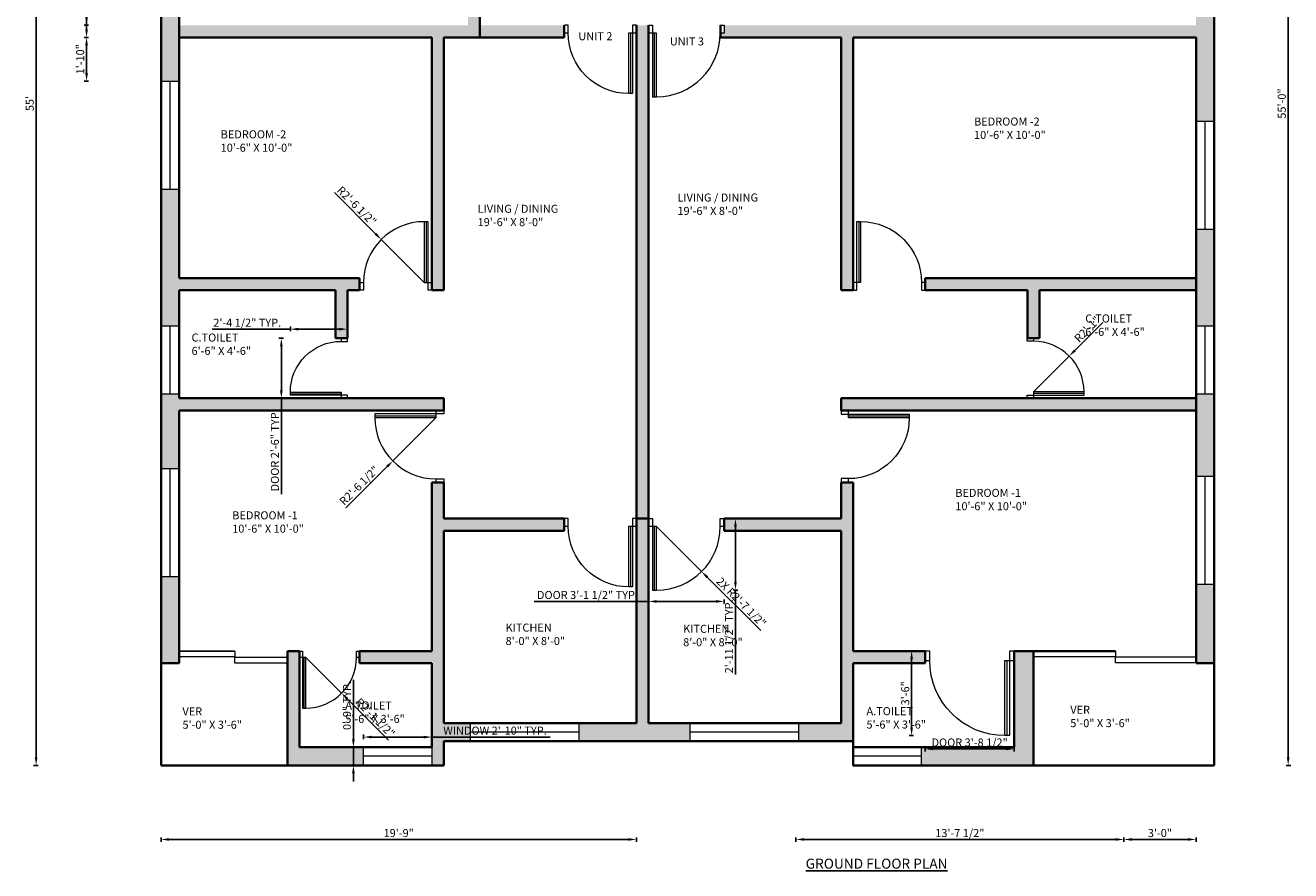
# Model space of a CAD drawing. Units: inches. Extents: x -66 to 565, y -698 to 61.
# Tile 1 of 2: x -66 to 565, y -698 to -276. Entities that reach past the tile are written whole.
import ezdxf

# ---------------------------------------------------------------- set-up
doc = ezdxf.new("R2010")
doc.units = ezdxf.units.IN
for name, color, linetype, lineweight in [('A-ANNO-DIMS', 2, 'Continuous', 18), ('A-ANNO-TEXT', 7, 'Continuous', 25), ('A-AREA-IDEN', 7, 'Continuous', 18), ('A-DOOR', 4, 'Continuous', 18), ('A-GLAZ', 111, 'Continuous', 18), ('A-WALL', 7, 'Continuous', 35), ('A-WALL-PATT', 252, 'Continuous', 13)]:
    doc.layers.add(name, color=color, linetype=linetype, lineweight=lineweight)
doc.styles.get("Standard").update_dxf_attribs({"font": 'arial.ttf'})
doc.dimstyles.new('ISO-25', dxfattribs={"dimtxt": 4, "dimasz": 4, "dimexe": 1.25, "dimexo": 0.625, "dimtad": 1, "dimlunit": 3, "dimtxsty": 'Standard', "dimcen": 2.5, "dimadec": 0, "dimazin": 0, "dimtfac": 1, "dimtmove": 0, "dimatfit": 3, "dimfxl": 1, "dimfxlon": 1, "dimarcsym": 0})

# ---------------------------------------------------------------- blocks, each defined once
blk = doc.blocks.new('A$C296830DC')
blk.add_line((829, 853), (829, 95))
for points in [[(853, 95), (853, 853), (805, 853), (805, 95)], [(47, 95), (47, 0), (0, 0), (0, 95)], [(900, 95), (900, 0), (853, 0), (853, 95)]]:
    blk.add_lwpolyline(points, close=True)
blk.add_arc((805, 95), 758, 90, 180)
blk = doc.blocks.new('*D3')
at = {"layer": 'A-ANNO-DIMS', "color": 0, "lineweight": -2, "transparency": 16777216}
for p, q in [((-59.68, 14.91), (-61.93, 14.91)), ((-60.68, 10.91), (-60.68, -641.09)), ((-59.68, -645.09), (-61.93, -645.09))]:
    blk.add_line(p, q, dxfattribs=at)
at = {"layer": 'A-ANNO-DIMS', "color": 0, "transparency": 16777216}
for points in [[(-61.35, 10.91), (-60.01, 10.91), (-60.68, 14.91)], [(-61.35, -641.09), (-60.01, -641.09), (-60.68, -645.09)]]:
    blk.add_solid(points, dxfattribs=at)
at = {"layer": 'Defpoints', "color": 0, "transparency": 16777216}
for p in [(1.61, 14.91), (-60.68, -645.09), (1.61, -645.09)]:
    blk.add_point(p, dxfattribs=at)
at = {"layer": 'A-ANNO-DIMS', "color": 0, "transparency": 16777216, "insert": (-63.34, -315.09), "char_height": 4, "attachment_point": 5, "rotation": 90}
blk.add_mtext("55'", dxfattribs=at)
blk = doc.blocks.new('WIN-54IN')
blk.add_line((4.5, 54), (4.5, 0))
blk.add_lwpolyline([(0, 54), (9, 54), (9, 0), (0, 0)], close=True)
blk = doc.blocks.new('WIN-34IN')
blk.add_line((34, 4.5), (0, 4.5))
blk.add_lwpolyline([(0, 9), (34, 9), (34, 0), (0, 0)], close=True)
blk = doc.blocks.new('*D8')
at = {"layer": 'A-ANNO-DIMS', "color": 0, "lineweight": -2, "transparency": 16777216}
for p, q in [((62.58, -432.1), (60.33, -432.1)), ((61.58, -436.1), (61.58, -458.14)), ((62.58, -462.14), (60.33, -462.14)), ((61.58, -462.14), (61.58, -509.89))]:
    blk.add_line(p, q, dxfattribs=at)
at = {"layer": 'A-ANNO-DIMS', "color": 0, "transparency": 16777216}
for points in [[(60.91, -436.1), (62.24, -436.1), (61.58, -432.1)], [(60.91, -458.14), (62.24, -458.14), (61.58, -462.14)]]:
    blk.add_solid(points, dxfattribs=at)
at = {"layer": 'Defpoints', "color": 0, "transparency": 16777216}
for p in [(66.08, -432.1), (61.58, -462.14), (66.08, -462.14)]:
    blk.add_point(p, dxfattribs=at)
at = {"layer": 'A-ANNO-DIMS', "color": 0, "transparency": 16777216, "insert": (58.88, -488.02), "char_height": 4, "attachment_point": 5, "rotation": 90}
blk.add_mtext('DOOR 2\'-6" TYP.', dxfattribs=at)
blk = doc.blocks.new('*D9')
at = {"layer": 'A-ANNO-DIMS', "color": 0, "lineweight": -2, "transparency": 16777216}
for p, q in [((66.08, -427.6), (27.06, -427.6)), ((66.08, -428.6), (66.08, -426.35)), ((90.54, -427.6), (70.08, -427.6)), ((94.54, -428.6), (94.54, -426.35))]:
    blk.add_line(p, q, dxfattribs=at)
at = {"layer": 'A-ANNO-DIMS', "color": 0, "transparency": 16777216}
for points in [[(70.08, -426.93), (70.08, -428.27), (66.08, -427.6)], [(90.54, -426.93), (90.54, -428.27), (94.54, -427.6)]]:
    blk.add_solid(points, dxfattribs=at)
at = {"layer": 'Defpoints', "color": 0, "transparency": 16777216}
for p in [(66.08, -427.6), (66.08, -432.1), (94.54, -432.1)]:
    blk.add_point(p, dxfattribs=at)
at = {"layer": 'A-ANNO-DIMS', "color": 0, "transparency": 16777216, "insert": (44.57, -424.91), "char_height": 4, "attachment_point": 5}
blk.add_mtext('2\'-4 1/2" TYP.', dxfattribs=at)
blk = doc.blocks.new('*D12')
at = {"layer": 'A-ANNO-DIMS', "color": 0, "lineweight": -2, "transparency": 16777216}
for p, q in [((244.73, -563.36), (187.66, -563.36)), ((244.73, -562.36), (244.73, -564.61)), ((278.34, -563.36), (248.73, -563.36)), ((282.34, -562.36), (282.34, -564.61))]:
    blk.add_line(p, q, dxfattribs=at)
at = {"layer": 'A-ANNO-DIMS', "color": 0, "transparency": 16777216}
for points in [[(248.73, -562.69), (248.73, -564.03), (244.73, -563.36)], [(278.34, -562.69), (278.34, -564.03), (282.34, -563.36)]]:
    blk.add_solid(points, dxfattribs=at)
at = {"layer": 'Defpoints', "color": 0, "transparency": 16777216}
for p in [(244.73, -557.72), (282.34, -557.72), (244.73, -563.36)]:
    blk.add_point(p, dxfattribs=at)
at = {"layer": 'A-ANNO-DIMS', "color": 0, "transparency": 16777216, "insert": (214.2, -560.66), "char_height": 4, "attachment_point": 5}
blk.add_mtext('DOOR 3\'-1 1/2" TYP.', dxfattribs=at)
blk = doc.blocks.new('*D13')
at = {"layer": 'A-ANNO-DIMS', "color": 0, "lineweight": -2, "transparency": 16777216}
for p, q in [((286.98, -522.09), (289.23, -522.09)), ((287.98, -526.09), (287.98, -553.72)), ((286.98, -557.72), (289.23, -557.72)), ((287.98, -557.72), (287.98, -599.85))]:
    blk.add_line(p, q, dxfattribs=at)
at = {"layer": 'A-ANNO-DIMS', "color": 0, "transparency": 16777216}
for points in [[(287.32, -526.09), (288.65, -526.09), (287.98, -522.09)], [(287.32, -553.72), (288.65, -553.72), (287.98, -557.72)]]:
    blk.add_solid(points, dxfattribs=at)
at = {"layer": 'Defpoints', "color": 0, "transparency": 16777216}
for p in [(282.34, -522.09), (282.34, -557.72), (287.98, -557.72)]:
    blk.add_point(p, dxfattribs=at)
at = {"layer": 'A-ANNO-DIMS', "color": 0, "transparency": 16777216, "insert": (285.29, -580.78), "char_height": 4, "attachment_point": 5, "rotation": 90}
blk.add_mtext('2\'-11 1/2" TYP.', dxfattribs=at)
blk = doc.blocks.new('*D14')
at = {"layer": 'A-ANNO-DIMS', "color": 0, "lineweight": -2, "transparency": 16777216}
for p, q in [((382.5, -635.91), (382.5, -638.16)), ((386.5, -636.91), (422.99, -636.91)), ((426.99, -635.91), (426.99, -638.16))]:
    blk.add_line(p, q, dxfattribs=at)
at = {"layer": 'A-ANNO-DIMS', "color": 0, "transparency": 16777216}
for points in [[(386.5, -636.24), (386.5, -637.58), (382.5, -636.91)], [(422.99, -636.24), (422.99, -637.58), (426.99, -636.91)]]:
    blk.add_solid(points, dxfattribs=at)
at = {"layer": 'Defpoints', "color": 0, "transparency": 16777216}
for p in [(382.5, -630.24), (426.99, -630.24), (426.99, -636.91)]:
    blk.add_point(p, dxfattribs=at)
at = {"layer": 'A-ANNO-DIMS', "color": 0, "transparency": 16777216, "insert": (404.74, -634.21), "char_height": 4, "attachment_point": 5}
blk.add_mtext('DOOR 3\'-8 1/2"', dxfattribs=at)
blk = doc.blocks.new('*D15')
at = {"layer": 'A-ANNO-DIMS', "color": 0, "lineweight": -2, "transparency": 16777216}
for p, q in [((376.82, -588.09), (374.57, -588.09)), ((375.82, -592.09), (375.82, -626.24)), ((376.82, -630.24), (374.57, -630.24))]:
    blk.add_line(p, q, dxfattribs=at)
at = {"layer": 'A-ANNO-DIMS', "color": 0, "transparency": 16777216}
for points in [[(375.16, -592.09), (376.49, -592.09), (375.82, -588.09)], [(375.16, -626.24), (376.49, -626.24), (375.82, -630.24)]]:
    blk.add_solid(points, dxfattribs=at)
at = {"layer": 'Defpoints', "color": 0, "transparency": 16777216}
for p in [(382.5, -588.09), (375.82, -630.24), (382.5, -630.24)]:
    blk.add_point(p, dxfattribs=at)
at = {"layer": 'A-ANNO-DIMS', "color": 0, "transparency": 16777216, "insert": (373.15, -609.16), "char_height": 4, "attachment_point": 5, "rotation": 90}
blk.add_mtext('3\'-6"', dxfattribs=at)
blk = doc.blocks.new('*D18')
at = {"layer": 'A-ANNO-DIMS', "color": 0, "lineweight": -2, "transparency": 16777216}
for p, q in [((102.6, -631.99), (102.6, -629.74)), ((136.6, -631.99), (136.6, -629.74)), ((106.6, -630.99), (132.6, -630.99)), ((136.6, -630.99), (195.57, -630.99))]:
    blk.add_line(p, q, dxfattribs=at)
at = {"layer": 'A-ANNO-DIMS', "color": 0, "transparency": 16777216}
for points in [[(106.6, -630.32), (106.6, -631.65), (102.6, -630.99)], [(132.6, -630.32), (132.6, -631.65), (136.6, -630.99)]]:
    blk.add_solid(points, dxfattribs=at)
at = {"layer": 'Defpoints', "color": 0, "transparency": 16777216}
for p in [(102.6, -636.09), (136.6, -630.99), (136.6, -636.09)]:
    blk.add_point(p, dxfattribs=at)
at = {"layer": 'A-ANNO-DIMS', "color": 0, "transparency": 16777216, "insert": (168.09, -628.29), "char_height": 4, "attachment_point": 5}
blk.add_mtext('WINDOW 2\'-10" TYP.', dxfattribs=at)
blk = doc.blocks.new('*D19')
at = {"layer": 'A-ANNO-DIMS', "color": 0, "lineweight": -2, "transparency": 16777216}
for p, q in [((97.5, -632.09), (97.5, -602.45)), ((98.5, -636.09), (96.25, -636.09)), ((97.5, -645.09), (97.5, -636.09)), ((98.5, -645.09), (96.25, -645.09)), ((97.5, -649.09), (97.5, -653.09))]:
    blk.add_line(p, q, dxfattribs=at)
at = {"layer": 'A-ANNO-DIMS', "color": 0, "transparency": 16777216}
for points in [[(96.83, -632.09), (98.17, -632.09), (97.5, -636.09)], [(96.83, -649.09), (98.17, -649.09), (97.5, -645.09)]]:
    blk.add_solid(points, dxfattribs=at)
at = {"layer": 'Defpoints', "color": 0, "transparency": 16777216}
for p in [(97.5, -636.09), (102.6, -636.09), (102.6, -645.09)]:
    blk.add_point(p, dxfattribs=at)
at = {"layer": 'A-ANNO-DIMS', "color": 0, "transparency": 16777216, "insert": (94.83, -615.27), "char_height": 4, "attachment_point": 5, "rotation": 90}
blk.add_mtext('0\'-9" TYP.', dxfattribs=at)
blk = doc.blocks.new('*D21')
at = {"layer": 'A-ANNO-DIMS', "color": 0, "lineweight": -2, "transparency": 16777216}
for p, q in [((562.56, 14.91), (564.81, 14.91)), ((563.56, 10.91), (563.56, -641.09)), ((562.56, -645.09), (564.81, -645.09))]:
    blk.add_line(p, q, dxfattribs=at)
at = {"layer": 'A-ANNO-DIMS', "color": 0, "transparency": 16777216}
for points in [[(562.89, 10.91), (564.23, 10.91), (563.56, 14.91)], [(562.89, -641.09), (564.23, -641.09), (563.56, -645.09)]]:
    blk.add_solid(points, dxfattribs=at)
at = {"layer": 'Defpoints', "color": 0, "transparency": 16777216}
for p in [(481.61, 14.91), (526.61, -645.09), (563.56, -645.09)]:
    blk.add_point(p, dxfattribs=at)
at = {"layer": 'A-ANNO-DIMS', "color": 0, "transparency": 16777216, "insert": (560.89, -315.09), "char_height": 4, "attachment_point": 5, "rotation": 90}
blk.add_mtext('55\'-0"', dxfattribs=at)
blk = doc.blocks.new('*D22')
at = {"layer": 'A-ANNO-DIMS', "color": 0, "lineweight": -2, "transparency": 16777216}
for p, q in [((-34.52, 14.91), (-36.77, 14.91)), ((-35.52, 10.91), (-35.52, -278.09)), ((-34.52, -282.09), (-36.77, -282.09))]:
    blk.add_line(p, q, dxfattribs=at)
at = {"layer": 'A-ANNO-DIMS', "color": 0, "transparency": 16777216}
for points in [[(-36.19, 10.91), (-34.86, 10.91), (-35.52, 14.91)], [(-36.19, -278.09), (-34.86, -278.09), (-35.52, -282.09)]]:
    blk.add_solid(points, dxfattribs=at)
at = {"layer": 'Defpoints', "color": 0, "transparency": 16777216}
for p in [(1.61, 14.91), (-35.52, -282.09), (10.61, -282.09)]:
    blk.add_point(p, dxfattribs=at)
at = {"layer": 'A-ANNO-DIMS', "color": 0, "transparency": 16777216, "insert": (-38.19, -133.59), "char_height": 4, "attachment_point": 5, "rotation": 90}
blk.add_mtext('24\'-9"', dxfattribs=at)
blk = doc.blocks.new('*D23')
at = {"layer": 'A-ANNO-DIMS', "color": 0, "lineweight": -2, "transparency": 16777216}
for p, q in [((1.61, -681.04), (1.61, -683.29)), ((238.61, -681.04), (238.61, -683.29)), ((5.61, -682.04), (234.61, -682.04))]:
    blk.add_line(p, q, dxfattribs=at)
at = {"layer": 'A-ANNO-DIMS', "color": 0, "transparency": 16777216}
for points in [[(5.61, -681.37), (5.61, -682.7), (1.61, -682.04)], [(234.61, -681.37), (234.61, -682.7), (238.61, -682.04)]]:
    blk.add_solid(points, dxfattribs=at)
at = {"layer": 'Defpoints', "color": 0, "transparency": 16777216}
for p in [(238.61, -624.09), (1.61, -645.09), (238.61, -682.04)]:
    blk.add_point(p, dxfattribs=at)
at = {"layer": 'A-ANNO-DIMS', "color": 0, "transparency": 16777216, "insert": (120.11, -679.37), "char_height": 4, "attachment_point": 5}
blk.add_mtext('19\'-9"', dxfattribs=at)
blk = doc.blocks.new('*D24')
at = {"layer": 'A-ANNO-DIMS', "color": 0, "lineweight": -2, "transparency": 16777216}
for p, q in [((-34.52, -186.09), (-36.77, -186.09)), ((-35.52, -190.09), (-35.52, -272.09)), ((-34.52, -276.09), (-36.77, -276.09))]:
    blk.add_line(p, q, dxfattribs=at)
at = {"layer": 'A-ANNO-DIMS', "color": 0, "transparency": 16777216}
for points in [[(-36.19, -190.09), (-34.86, -190.09), (-35.52, -186.09)], [(-36.19, -272.09), (-34.86, -272.09), (-35.52, -276.09)]]:
    blk.add_solid(points, dxfattribs=at)
at = {"layer": 'Defpoints', "color": 0, "transparency": 16777216}
for p in [(318.11, -186.09), (-35.52, -276.09), (318.11, -276.09)]:
    blk.add_point(p, dxfattribs=at)
at = {"layer": 'A-ANNO-DIMS', "color": 0, "transparency": 16777216, "insert": (-38.19, -231.09), "char_height": 4, "attachment_point": 5, "rotation": 90}
blk.add_mtext('7\'-6"', dxfattribs=at)
blk = doc.blocks.new('*D25')
at = {"layer": 'A-ANNO-DIMS', "color": 0, "lineweight": -2, "transparency": 16777216}
for p, q in [((318.11, -681.04), (318.11, -683.29)), ((481.61, -681.04), (481.61, -683.29)), ((322.11, -682.04), (477.61, -682.04))]:
    blk.add_line(p, q, dxfattribs=at)
at = {"layer": 'A-ANNO-DIMS', "color": 0, "transparency": 16777216}
for points in [[(322.11, -681.37), (322.11, -682.7), (318.11, -682.04)], [(477.61, -681.37), (477.61, -682.7), (481.61, -682.04)]]:
    blk.add_solid(points, dxfattribs=at)
at = {"layer": 'Defpoints', "color": 0, "transparency": 16777216}
for p in [(318.11, -276.09), (481.61, -276.09), (481.61, -682.04)]:
    blk.add_point(p, dxfattribs=at)
at = {"layer": 'A-ANNO-DIMS', "color": 0, "transparency": 16777216, "insert": (399.86, -679.34), "char_height": 4, "attachment_point": 5}
blk.add_mtext('13\'-7 1/2"', dxfattribs=at)
blk = doc.blocks.new('*D26')
at = {"layer": 'A-ANNO-DIMS', "color": 0, "lineweight": -2, "transparency": 16777216}
for p, q in [((481.61, -681.04), (481.61, -683.29)), ((517.61, -681.04), (517.61, -683.29)), ((513.61, -682.04), (485.61, -682.04))]:
    blk.add_line(p, q, dxfattribs=at)
at = {"layer": 'A-ANNO-DIMS', "color": 0, "transparency": 16777216}
for points in [[(485.61, -681.37), (485.61, -682.7), (481.61, -682.04)], [(513.61, -681.37), (513.61, -682.7), (517.61, -682.04)]]:
    blk.add_solid(points, dxfattribs=at)
at = {"layer": 'Defpoints', "color": 0, "transparency": 16777216}
for p in [(481.61, -276.09), (517.61, -276.09), (481.61, -682.04)]:
    blk.add_point(p, dxfattribs=at)
at = {"layer": 'A-ANNO-DIMS', "color": 0, "transparency": 16777216, "insert": (499.61, -679.37), "char_height": 4, "attachment_point": 5}
blk.add_mtext('3\'-0"', dxfattribs=at)
blk = doc.blocks.new('*D28')
at = {"layer": 'A-ANNO-DIMS', "color": 0, "lineweight": -2, "transparency": 16777216}
for p, q in [((-34.52, -282.09), (-36.77, -282.09)), ((-35.52, -286.09), (-35.52, -299.95)), ((-34.52, -303.95), (-36.77, -303.95))]:
    blk.add_line(p, q, dxfattribs=at)
at = {"layer": 'A-ANNO-DIMS', "color": 0, "transparency": 16777216}
for points in [[(-36.19, -286.09), (-34.86, -286.09), (-35.52, -282.09)], [(-36.19, -299.95), (-34.86, -299.95), (-35.52, -303.95)]]:
    blk.add_solid(points, dxfattribs=at)
at = {"layer": 'Defpoints', "color": 0, "transparency": 16777216}
for p in [(10.61, -282.09), (-35.52, -303.95), (1.55, -303.95)]:
    blk.add_point(p, dxfattribs=at)
at = {"layer": 'A-ANNO-DIMS', "color": 0, "transparency": 16777216, "insert": (-38.19, -293.02), "char_height": 4, "attachment_point": 5, "rotation": 90}
blk.add_mtext('1\'-10"', dxfattribs=at)
blk = doc.blocks.new('*D29')
at = {"layer": 'A-ANNO-DIMS', "color": 0, "lineweight": -2, "transparency": 16777216}
for p, q in [((248.69, -526.04), (271.09, -548.44)), ((300.57, -577.92), (273.91, -551.27))]:
    blk.add_line(p, q, dxfattribs=at)
at = {"layer": 'A-ANNO-DIMS', "color": 0, "transparency": 16777216}
blk.add_solid([(274.39, -550.8), (273.44, -551.74), (271.09, -548.44)], dxfattribs=at)
at = {"layer": 'Defpoints', "color": 0, "transparency": 16777216}
for p in [(248.69, -526.04), (271.09, -548.44)]:
    blk.add_point(p, dxfattribs=at)
at = {"layer": 'A-ANNO-DIMS', "color": 0, "transparency": 16777216, "insert": (290.56, -564.11), "char_height": 4, "attachment_point": 5, "rotation": 315.00012}
blk.add_mtext('2X R2\'-7 1/2"', dxfattribs=at)
blk = doc.blocks.new('*D30')
at = {"layer": 'A-ANNO-DIMS', "color": 0, "lineweight": -2, "transparency": 16777216}
for p, q in [((138.76, -471.7), (117.16, -493.31)), ((93.8, -516.66), (114.33, -496.14))]:
    blk.add_line(p, q, dxfattribs=at)
at = {"layer": 'A-ANNO-DIMS', "color": 0, "transparency": 16777216}
blk.add_solid([(113.86, -495.66), (114.8, -496.61), (117.16, -493.31)], dxfattribs=at)
at = {"layer": 'Defpoints', "color": 0, "transparency": 16777216}
for p in [(138.76, -471.7), (117.16, -493.31)]:
    blk.add_point(p, dxfattribs=at)
at = {"layer": 'A-ANNO-DIMS', "color": 0, "transparency": 16777216, "insert": (100.74, -505.91), "char_height": 4, "attachment_point": 5, "rotation": 45.00091}
blk.add_mtext('R2\'-6 1/2"', dxfattribs=at)
blk = doc.blocks.new('*D33')
at = {"layer": 'A-ANNO-DIMS', "color": 0, "lineweight": -2, "transparency": 16777216}
for p, q in [((88.05, -359.53), (108.58, -380.06)), ((132.82, -404.3), (111.41, -382.89))]:
    blk.add_line(p, q, dxfattribs=at)
at = {"layer": 'A-ANNO-DIMS', "color": 0, "transparency": 16777216}
blk.add_solid([(109.05, -379.59), (108.11, -380.53), (111.41, -382.89)], dxfattribs=at)
at = {"layer": 'Defpoints', "color": 0, "transparency": 16777216}
for p in [(111.41, -382.89), (132.82, -404.3)]:
    blk.add_point(p, dxfattribs=at)
at = {"layer": 'A-ANNO-DIMS', "color": 0, "transparency": 16777216, "insert": (98.81, -366.48), "char_height": 4, "attachment_point": 5, "rotation": 315.00004}
blk.add_mtext('R2\'-6 1/2"', dxfattribs=at)
blk = doc.blocks.new('*D36')
at = {"layer": 'A-ANNO-DIMS', "color": 0, "lineweight": -2, "transparency": 16777216}
for p, q in [((73.77, -591.24), (91.63, -609.1)), ((114.98, -632.46), (94.45, -611.93))]:
    blk.add_line(p, q, dxfattribs=at)
at = {"layer": 'A-ANNO-DIMS', "color": 0, "transparency": 16777216}
blk.add_solid([(94.93, -611.46), (93.98, -612.4), (91.63, -609.1)], dxfattribs=at)
at = {"layer": 'Defpoints', "color": 0, "transparency": 16777216}
for p in [(73.77, -591.24), (91.63, -609.1)]:
    blk.add_point(p, dxfattribs=at)
at = {"layer": 'A-ANNO-DIMS', "color": 0, "transparency": 16777216, "insert": (108.04, -621.71), "char_height": 4, "attachment_point": 5, "rotation": 314.99996}
blk.add_mtext('R2\'-1 1/2"', dxfattribs=at)
blk = doc.blocks.new('*D37')
at = {"layer": 'A-ANNO-DIMS', "color": 0, "lineweight": -2, "transparency": 16777216}
for p, q in [((471.14, -424.26), (457.21, -438.2)), ((436.56, -458.84), (454.38, -441.02))]:
    blk.add_line(p, q, dxfattribs=at)
at = {"layer": 'A-ANNO-DIMS', "color": 0, "transparency": 16777216}
blk.add_solid([(456.73, -437.72), (457.68, -438.67), (454.38, -441.02)], dxfattribs=at)
at = {"layer": 'Defpoints', "color": 0, "transparency": 16777216}
for p in [(454.38, -441.02), (436.56, -458.84)]:
    blk.add_point(p, dxfattribs=at)
at = {"layer": 'A-ANNO-DIMS', "color": 0, "transparency": 16777216, "insert": (463.73, -427.95), "char_height": 4, "attachment_point": 5, "rotation": 45.0011}
blk.add_mtext('R2\'-1"', dxfattribs=at)

msp = doc.modelspace()

# ---------------------------------------------------------------- hatches: boundary and pattern name
at = {"layer": 'A-WALL-PATT'}
h = msp.add_hatch(color=256, dxfattribs=at)
h.dxf.hatch_style = 1
h.paths.add_polyline_path([(53.054, 14.914), (1.609, 14.914), (1.609, -25.926), (10.609, -25.926), (10.609, 5.914), (53.054, 5.914)])
h.paths.add_polyline_path([(174.609, 14.914), (107.054, 14.914), (107.054, 5.914), (154.609, 5.914), (154.609, -132.086), (160.609, -132.086), (160.609, -84.086), (178.441, -84.086), (178.441, -80.91), (178.609, -78.086), (160.609, -78.086), (160.609, 5.914), (174.609, 5.914)])
h.paths.add_polyline_path([(357.494, 14.914), (275.363, 14.914), (275.363, 5.914), (286.609, 5.914), (286.609, -78.086), (250.609, -78.086), (250.609, -84.086), (286.609, -84.086), (286.609, -89.827), (290.425, -89.827), (290.425, -90.086), (292.609, -90.086), (292.609, 5.914), (357.494, 5.914)])
h.paths.add_polyline_path([(221.363, 14.914), (208.609, 14.914), (208.609, 5.914), (208.609, -84.086), (214.609, -84.086), (214.609, 5.914), (221.363, 5.914)])
h.paths.add_polyline_path([(481.609, 14.914), (411.494, 14.914), (411.494, 5.914), (472.609, 5.914), (472.609, -30.057), (477.316, -30.057), (481.609, -30.057)])
h.paths.add_polyline_path([(481.609, -94.45), (472.609, -94.45), (472.609, -126.086), (376.678, -126.086), (376.678, -129.244), (376.609, -132.086), (472.609, -132.086), (472.609, -180.086), (154.609, -180.086), (154.609, -186.086), (481.609, -186.086), (517.609, -186.086), (517.609, -209.408), (526.609, -209.408), (526.609, -180.086), (523.609, -180.086), (481.609, -180.086)])
h.paths.add_polyline_path([(346.609, -126.086), (292.609, -126.086), (286.609, -126.086), (286.609, -132.086), (292.609, -132.086), (346.609, -132.086)], flags=17)
h.paths.add_polyline_path([(118.491, -128.284), (118.609, -126.086), (10.609, -126.086), (10.609, -132.086), (118.491, -132.086)])
h.paths.add_polyline_path([(10.609, -79.926), (1.609, -79.926), (1.609, -171.746), (10.609, -171.746)])
h.paths.add_polyline_path([(10.609, -225.746), (1.609, -225.746), (1.609, -303.953), (10.609, -303.953)])
h.paths.add_polyline_path([(160.609, -222.168), (156.831, -222.168), (154.609, -222.086), (154.609, -276.086), (10.609, -276.086), (10.609, -282.086), (136.609, -282.086), (136.609, -408.086), (142.609, -408.086), (142.609, -282.086), (160.609, -282.086)])
h.paths.add_polyline_path([(202.609, -276.086), (160.609, -276.086), (160.609, -282.086), (202.609, -282.086)])
h.paths.add_polyline_path([(526.609, -263.408), (517.609, -263.408), (517.609, -276.086), (282.342, -276.086), (282.342, -280.017), (280.606, -280.017), (280.606, -282.086), (340.609, -282.086), (340.609, -408.086), (346.609, -408.086), (346.609, -404.294), (346.609, -282.086), (517.609, -282.086), (517.609, -323.855), (526.609, -323.855), (526.609, -282.086)])
h.paths.add_polyline_path([(244.609, -276.086), (238.609, -276.086), (238.609, -279.866), (238.609, -522.086), (244.609, -522.086)])
h.paths.add_polyline_path([(526.609, -377.855), (517.609, -377.855), (517.609, -425.984), (526.609, -425.984)])
h.paths.add_polyline_path([(517.609, -402.086), (382.609, -402.086), (382.609, -404.294), (382.631, -404.294), (382.631, -408.086), (433.609, -408.086), (433.609, -432.07), (436.561, -432.07), (439.609, -432.086), (439.609, -408.086), (517.609, -408.086)])
h.paths.add_polyline_path([(517.609, -462.086), (439.609, -462.086), (340.609, -462.086), (340.609, -468.086), (344.391, -468.086), (439.609, -468.086), (517.609, -468.086)])
h.paths.add_polyline_path([(526.609, -459.984), (517.609, -459.984), (517.609, -500.965), (526.609, -500.965)])
h.paths.add_polyline_path([(526.609, -554.965), (517.609, -554.965), (517.609, -594.086), (526.609, -594.086)])
h.paths.add_polyline_path([(436.609, -588.086), (426.99, -588.086), (426.99, -592.769), (426.99, -636.086), (380.508, -636.086), (380.508, -645.086), (436.609, -645.086)])
h.paths.add_polyline_path([(346.609, -504.086), (340.609, -504.086), (340.609, -522.086), (282.342, -522.086), (282.342, -526.045), (282.342, -528.086), (340.609, -528.086), (340.609, -624.086), (319.481, -624.086), (319.481, -633.086), (346.609, -633.086), (346.609, -594.086), (382.609, -594.086), (382.609, -592.769), (382.497, -592.769), (382.497, -588.086), (346.609, -588.086)])
h.paths.add_polyline_path([(265.481, -624.086), (244.609, -624.086), (244.609, -522.086), (238.609, -522.086), (238.609, -624.086), (209.858, -624.086), (209.858, -633.086), (265.481, -633.086)])
h.paths.add_polyline_path([(142.609, -528.086), (202.609, -528.086), (202.609, -522.086), (142.609, -522.086), (142.609, -504.167), (138.764, -504.167), (136.609, -504.086), (136.609, -588.086), (100.609, -588.086), (100.609, -594.086), (136.609, -594.086), (136.609, -636.086), (136.6, -636.086), (136.6, -645.086), (142.609, -645.086), (142.609, -633.086), (155.858, -633.086), (155.858, -624.086), (142.609, -624.086), (142.609, -588.086)])
h.paths.add_polyline_path([(102.6, -636.086), (70.609, -636.086), (70.609, -588.086), (64.609, -588.086), (64.609, -645.086), (70.609, -645.086), (102.6, -645.086)])
h.paths.add_polyline_path([(10.609, -551.068), (1.609, -551.068), (1.609, -594.086), (10.609, -594.086)])
h.paths.add_polyline_path([(10.609, -468.086), (88.609, -468.086), (138.764, -468.086), (138.764, -467.878), (142.609, -467.878), (142.609, -462.086), (94.536, -462.086), (94.536, -462.142), (91.375, -462.142), (88.609, -462.086), (10.609, -462.086), (10.609, -459.984), (1.609, -459.984), (1.609, -497.068), (10.609, -497.068)])
h.paths.add_polyline_path([(100.609, -402.086), (10.609, -402.086), (10.609, -357.953), (1.609, -357.953), (1.609, -425.984), (10.609, -425.984), (10.609, -408.086), (88.609, -408.086), (88.609, -432.086), (94.609, -432.086), (94.609, -408.086), (100.609, -408.086)])

# ---------------------------------------------------------------- linework, layer by layer
at = {"layer": 'A-DOOR'}
for p, q in [((38.329, -588.086), (10.609, -588.086)), ((64.609, -594.086), (38.324, -594.086))]:
    msp.add_line(p, q, dxfattribs=at)
for points in [[(10.609, -588.086), (38.329, -588.086), (38.329, -591.022), (10.609, -591.022)], [(436.609, -588.086), (477.514, -588.086), (477.514, -591.051), (436.609, -591.051)]]:
    msp.add_lwpolyline(points, close=True, dxfattribs=at)
for points in [[(64.609, -594.086), (38.324, -594.086), (38.324, -591.149), (64.609, -591.149)], [(517.609, -594.016), (477.514, -594.016), (477.514, -591.051), (517.609, -591.051)]]:
    msp.add_lwpolyline(points, dxfattribs=at)
at = {"layer": 'A-WALL'}
for p, q in [((1.609, -645.086), (1.609, 14.914)), ((10.609, -402.086), (10.609, 5.914)), ((526.609, -180.086), (526.609, -282.086)), ((160.609, -282.086), (160.609, -222.086)), ((202.609, -282.086), (202.609, -276.086)), ((238.609, -276.086), (238.609, -624.086)), ((244.609, -276.086), (244.609, -624.086)), ((280.606, -282.086), (280.606, -276.086)), ((136.609, -282.086), (10.609, -282.086)), ((136.609, -282.086), (136.609, -408.086)), ((142.609, -282.086), (142.609, -408.086)), ((202.609, -282.086), (142.609, -282.086)), ((340.609, -282.086), (280.606, -282.086)), ((340.609, -282.086), (340.609, -408.086)), ((517.609, -282.086), (346.609, -282.086)), ((346.609, -282.086), (346.609, -408.086)), ((517.609, -282.086), (517.609, -594.086)), ((526.609, -282.086), (526.609, -645.086)), ((100.609, -402.086), (10.609, -402.086)), ((100.609, -402.086), (100.609, -408.086)), ((517.609, -402.086), (382.609, -402.086)), ((382.609, -408.086), (382.609, -402.086)), ((10.609, -462.086), (10.609, -408.086)), ((88.609, -408.086), (10.609, -408.086)), ((88.609, -408.086), (88.609, -432.086)), ((100.609, -408.086), (94.609, -408.086)), ((94.609, -408.086), (94.609, -432.086)), ((136.609, -408.086), (142.609, -408.086)), ((346.609, -408.086), (340.609, -408.086)), ((433.609, -408.086), (382.609, -408.086)), ((433.609, -408.086), (433.609, -432.086)), ((517.609, -408.086), (439.609, -408.086)), ((439.609, -408.086), (439.609, -432.086)), ((94.609, -432.086), (88.609, -432.086)), ((439.609, -432.086), (433.609, -432.086)), ((88.609, -462.086), (10.609, -462.086)), ((88.609, -462.086), (142.609, -462.086)), ((142.609, -462.086), (142.609, -468.086)), ((439.609, -462.086), (340.609, -462.086)), ((340.609, -462.086), (340.609, -468.086)), ((439.609, -462.086), (517.609, -462.086)), ((88.609, -468.086), (10.609, -468.086)), ((10.609, -594.086), (10.609, -468.086)), ((88.609, -468.086), (120.086, -468.086)), ((88.609, -468.086), (142.609, -468.086)), ((439.609, -468.086), (340.609, -468.086)), ((439.609, -468.086), (517.609, -468.086)), ((136.609, -588.086), (136.609, -504.086)), ((136.609, -504.086), (142.609, -504.086)), ((142.609, -522.086), (142.609, -504.086)), ((346.609, -504.086), (340.609, -504.086)), ((340.609, -504.086), (340.609, -522.086)), ((346.609, -504.086), (346.609, -588.086)), ((202.609, -522.086), (142.609, -522.086)), ((202.609, -522.086), (202.609, -528.086)), ((238.609, -522.086), (244.609, -522.086)), ((340.609, -522.086), (282.342, -522.086)), ((282.342, -528.086), (282.342, -522.086)), ((142.609, -588.086), (142.609, -528.086)), ((202.609, -528.086), (142.609, -528.086)), ((340.609, -528.086), (282.342, -528.086)), ((340.609, -528.086), (340.609, -624.086)), ((70.609, -588.086), (64.609, -588.086)), ((64.609, -588.086), (64.609, -645.086)), ((70.609, -588.086), (70.609, -636.086)), ((100.609, -588.086), (136.609, -588.086)), ((100.609, -594.086), (100.609, -588.086)), ((142.609, -588.086), (142.609, -624.086)), ((346.609, -588.086), (382.609, -588.086)), ((382.609, -594.086), (382.609, -588.086)), ((426.99, -588.086), (426.99, -636.086)), ((426.99, -588.086), (477.514, -588.086)), ((436.609, -588.086), (436.609, -645.086)), ((10.609, -594.086), (1.609, -594.086)), ((100.609, -594.086), (136.609, -594.086)), ((136.609, -594.086), (136.609, -636.086)), ((346.609, -594.086), (382.609, -594.086)), ((346.609, -594.086), (346.609, -645.086)), ((517.609, -594.086), (526.609, -594.086)), ((238.609, -624.086), (142.609, -624.086)), ((340.609, -624.086), (244.609, -624.086)), ((70.609, -636.086), (136.609, -636.086)), ((346.609, -633.086), (142.609, -633.086)), ((142.609, -633.086), (142.609, -645.086)), ((346.609, -636.086), (426.99, -636.086)), ((10.609, -645.086), (1.609, -645.086)), ((10.609, -645.086), (70.609, -645.086)), ((70.609, -645.086), (142.609, -645.086)), ((346.609, -645.086), (526.609, -645.086))]:
    msp.add_line(p, q, dxfattribs=at)

# ---------------------------------------------------------------- block references
at = {"layer": 'A-DOOR'}
for p, xscale, yscale, zscale, rotation in [((202.697, -276.086), -0.0399020096887821, 0.0399020096887821, 0.0399020096887821, 180), ((282.342, -276.058), 0.0417895516625183, 0.0417895516625183, 0.0417895516625183, 180), ((94.536, -432.105), -0.0333742298353017, 0.0333742298353017, 0.0333742298353017, 90), ((433.412, -432.07), 0.0332445548126588, 0.0332445548126588, 0.0332445548126588, 270), ((142.584, -504.167), 0.040321223230596, 0.040321223230596, 0.040321223230596, 90), ((340.609, -504.018), -0.0399250848014763, 0.0399250848014763, 0.0399250848014763, 270), ((202.697, -522.086), -0.0399020096887821, 0.0399020096887821, 0.0399020096887821, 180), ((282.342, -522.086), 0.0417895516625183, 0.0417895516625183, 0.0417895516625183, 180), ((100.602, -588.086), 0.0333263621181619, 0.0333263621181619, 0.0333263621181619, 180), ((382.497, -588.086), -0.0494365581358181, 0.0494365581358181, 0.0494365581358181, 180)]:
    msp.add_blockref('A$C296830DC', p, dxfattribs=dict(at, xscale=xscale, yscale=yscale, zscale=zscale, rotation=rotation))
for p, xscale, yscale, zscale in [((100.649, -408.086), 0.039955163613067, 0.039955163613067, 0.039955163613067), ((382.631, -408.086), -0.0400252553789313, 0.0400252553789313, 0.0400252553789313)]:
    msp.add_blockref('A$C296830DC', p, dxfattribs=dict(at, xscale=xscale, yscale=yscale, zscale=zscale))
at = {"layer": 'A-GLAZ'}
for name, p in [('WIN-54IN', (1.554, -357.953)), ('WIN-54IN', (517.579, -377.855)), ('WIN-54IN', (1.496, -551.068)), ('WIN-54IN', (517.519, -554.965)), ('WIN-34IN', (102.6, -645.086)), ('WIN-34IN', (346.508, -645.086))]:
    msp.add_blockref(name, p, dxfattribs=at)
for name, p, rotation in [('WIN-34IN', (1.608, -425.984), 269.9999999999998), ('WIN-34IN', (517.608, -425.984), 270), ('WIN-54IN', (155.858, -624.086), 270), ('WIN-54IN', (265.481, -624.086), 270.0000000000002)]:
    msp.add_blockref(name, p, dxfattribs=dict(at, rotation=rotation))

# ---------------------------------------------------------------- texts
at = {"layer": 'A-ANNO-TEXT', "insert": (323, -691.617), "char_height": 5, "attachment_point": 1}
msp.add_mtext_dynamic_manual_height_columns('{\\fArial|b1|i0|c0|p34;\\LGROUND FLOOR PLAN}', width=410.76337, gutter_width=12.5, heights=[0], dxfattribs=at)
at = {"layer": 'A-AREA-IDEN', "char_height": 4, "attachment_point": 1}
for s, width, insert in [('UNIT 2', 21.86701, (209.657, -279.542)), ('UNIT 3', 36.68015, (255.272, -282.126)), ('BEDROOM -2\\P10\'-6" X 10\'-0"', 118.12834, (406.95, -322.078)), ('BEDROOM -2\\P10\'-6" X 10\'-0"', 85.4311, (31.341, -328.458)), ('LIVING / DINING\\P19\'-6" X 8\'-0"', 55.79354, (159.456, -365.568)), ('LIVING / DINING\\P19\'-6" X 8\'-0"', 56.16799, (259.061, -359.956)), ('C.TOILET\\P6\'-6" X 4\'-6"', 42.79473, (462.375, -420.278)), ('C.TOILET\\P6\'-6" X 4\'-6"', 43.82866, (16.809, -429.772)), ('BEDROOM -1\\P10\'-6" X 10\'-0"', 99.56183, (397.613, -507.218)), ('BEDROOM -1\\P10\'-6" X 10\'-0"', 71.07736, (37.099, -518.419)), ('KITCHEN\\P8\'-0" X 8\'-0"', 64.5168, (173.379, -574.408)), ('KITCHEN\\P8\'-0" X 8\'-0"', 53.45677, (261.921, -575.008)), ('VER\\P5\'-0" X 3\'-6"', 34.91449, (12.284, -616.185)), ('A.TOILET\\P5\'-6" X 3\'-6"', 33.26647, (93.46, -613.262)), ('A.TOILET\\P5\'-6" X 3\'-6"', 51.39213, (353.311, -616.076)), ('VER\\P5\'-0" X 3\'-6"', 48.84567, (454.938, -615.382))]:
    msp.add_mtext_dynamic_manual_height_columns(s, width=width, gutter_width=12.5, heights=[0], dxfattribs=dict(at, insert=insert))

# ---------------------------------------------------------------- dimensions: what is measured, and where the dimension line sits
at = {"layer": 'A-ANNO-DIMS'}
for base, p1, p2, angle, override, picture, middle in [((-60.681, -645.086), (1.609, 14.914), (1.609, -645.086), 90, {"dimclrd": 0, "dimclre": 0, "dimclrt": 0}, '*D3', (-63.34, -315.086)), ((-35.523, -282.086), (1.609, 14.914), (10.609, -282.086), 90, {"dimdec": 1, "dimlfac": 1, "dimrnd": 0, "dimzin": 1, "dimdsep": 46, "dimlunit": 4, "dimfrac": 2}, '*D22', (-38.19, -133.586)), ((563.559, -645.086), (481.609, 14.914), (526.609, -645.086), 90, {"dimdec": 1, "dimlfac": 1, "dimrnd": 0, "dimzin": 1, "dimdsep": 46, "dimlunit": 4, "dimfrac": 2}, '*D21', (560.891, -315.086)), ((-35.523, -276.086), (318.109, -186.086), (318.109, -276.086), 90, {"dimdec": 1, "dimlfac": 1, "dimrnd": 0, "dimzin": 1, "dimdsep": 46, "dimlunit": 4, "dimfrac": 2}, '*D24', (-38.19, -231.086)), ((-35.523, -303.953), (10.609, -282.086), (1.554, -303.953), 90, {"dimdec": 1, "dimlfac": 1, "dimrnd": 0, "dimzin": 1, "dimdsep": 46, "dimlunit": 4, "dimfrac": 2}, '*D28', (-38.19, -293.019)), ((375.823, -630.237), (382.497, -588.086), (382.497, -630.237), 270, {"dimdec": 1, "dimlfac": 1, "dimrnd": 0, "dimzin": 1, "dimdsep": 46, "dimlunit": 4, "dimfrac": 2}, '*D15', (373.154, -609.161))]:
    dim = msp.add_linear_dim(base=base, p1=p1, p2=p2, angle=angle, dimstyle='ISO-25', override=override, dxfattribs=at)
    dim.commit()
    dim.dimension.update_dxf_attribs({"geometry": picture, "text_midpoint": middle})
for base, p1, p2, picture, middle in [((481.609, -682.036), (318.109, -276.086), (481.609, -276.086), '*D25', (399.859, -679.341)), ((481.609, -682.036), (517.609, -276.086), (481.609, -276.086), '*D26', (499.609, -679.367)), ((238.609, -682.036), (1.609, -645.086), (238.609, -624.086), '*D23', (120.109, -679.368))]:
    dim = msp.add_linear_dim(base=base, p1=p1, p2=p2, dimstyle='ISO-25', override={"dimdec": 1, "dimlfac": 1, "dimrnd": 0, "dimzin": 1, "dimdsep": 46, "dimlunit": 4, "dimfrac": 2}, dxfattribs=at)
    dim.commit()
    dim.dimension.update_dxf_attribs({"geometry": picture, "text_midpoint": middle})
for center, mpoint, picture, middle in [((132.823, -404.3), (111.411, -382.888), '*D33', (98.808, -366.477)), ((436.561, -458.841), (454.377, -441.024), '*D37', (463.726, -427.95)), ((138.764, -471.698), (117.156, -493.307), '*D30', (100.745, -505.91)), ((73.766, -591.243), (91.626, -609.103), '*D36', (108.037, -621.705))]:
    dim = msp.add_radius_dim(center=center, mpoint=mpoint, dimstyle='ISO-25', override={"dimdec": 1, "dimlfac": 1, "dimrnd": 0, "dimzin": 1, "dimdsep": 46, "dimlunit": 4, "dimfrac": 2}, dxfattribs=at)
    dim.commit()
    dim.dimension.update_dxf_attribs({"geometry": picture, "text_midpoint": middle})
for base, p1, p2, angle, text, picture, middle in [((66.081, -427.599), (94.536, -432.105), (66.081, -432.105), 180, '<> TYP.', '*D9', (44.57, -424.906)), ((61.575, -462.142), (66.081, -432.105), (66.081, -462.142), 270, 'DOOR <> TYP.', '*D8', (58.88, -488.016)), ((287.984, -557.717), (282.342, -522.086), (282.342, -557.717), 270, '<> TYP.', '*D13', (285.291, -580.781)), ((244.732, -563.358), (282.342, -557.717), (244.732, -557.717), 180, 'DOOR <> TYP.', '*D12', (214.197, -560.662)), ((97.5, -636.086), (102.6, -645.086), (102.6, -636.086), 90, '<> TYP.', '*D19', (94.833, -615.27))]:
    dim = msp.add_linear_dim(base=base, p1=p1, p2=p2, angle=angle, text=text, dimstyle='ISO-25', override={"dimdec": 1, "dimlfac": 1, "dimrnd": 0, "dimzin": 1, "dimdsep": 46, "dimlunit": 4, "dimfrac": 2}, dxfattribs=at)
    dim.commit()
    dim.dimension.update_dxf_attribs({"geometry": picture, "text_midpoint": middle})
dim = msp.add_radius_dim(center=(248.691, -526.045), mpoint=(271.086, -548.44), text='2X <>', dimstyle='ISO-25', override={"dimdec": 1, "dimlfac": 1, "dimrnd": 0, "dimzin": 1, "dimdsep": 46, "dimlunit": 4, "dimfrac": 2}, dxfattribs=at)
dim.commit()
dim.dimension.update_dxf_attribs({"geometry": '*D29', "text_midpoint": (290.56, -564.106)})
for base, p1, p2, text, picture, middle in [((136.6, -630.986), (102.6, -636.086), (136.6, -636.086), 'WINDOW <> TYP.', '*D18', (168.087, -628.291)), ((426.99, -636.911), (382.497, -630.237), (426.99, -630.237), 'DOOR <>', '*D14', (404.743, -634.215))]:
    dim = msp.add_linear_dim(base=base, p1=p1, p2=p2, text=text, dimstyle='ISO-25', override={"dimdec": 1, "dimlfac": 1, "dimrnd": 0, "dimzin": 1, "dimdsep": 46, "dimlunit": 4, "dimfrac": 2}, dxfattribs=at)
    dim.commit()
    dim.dimension.update_dxf_attribs({"geometry": picture, "text_midpoint": middle})

doc.saveas('drawing.dxf')
